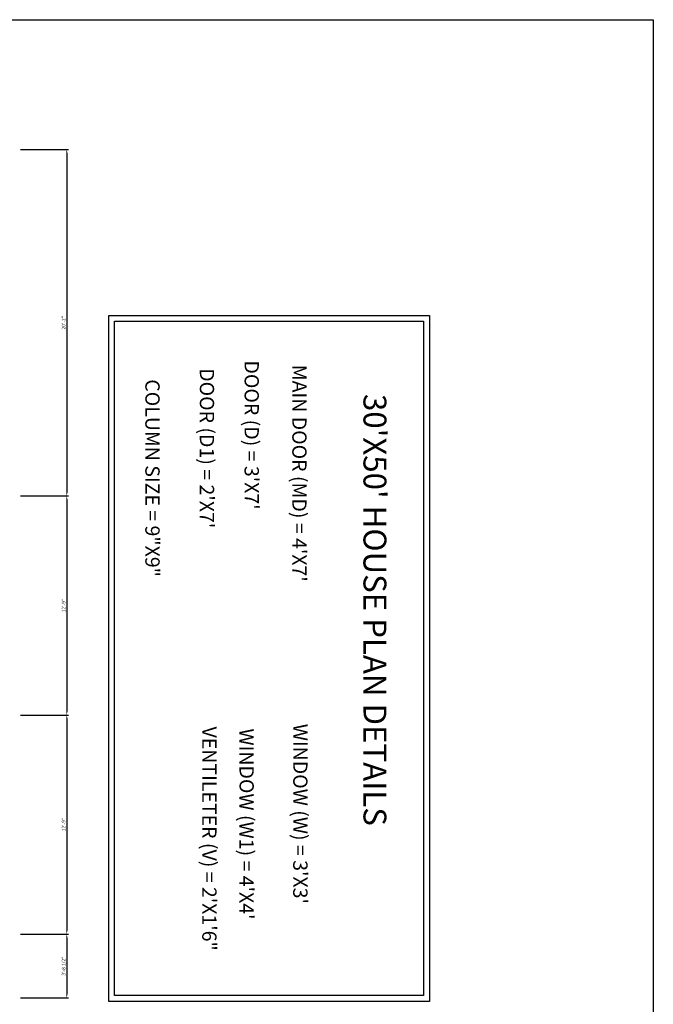
# Model space of a CAD drawing. Units: inches. Extents: x 2163 to 7246, y 928 to 2098.
# Tile 10 of 15: x 3191 to 3633, y 1411 to 2098. Entities that reach past the tile are written whole.
import ezdxf

# ---------------------------------------------------------------- set-up
doc = ezdxf.new("R2010")
doc.units = ezdxf.units.IN
for name, color, linetype, lineweight in [('A-ANNO-DIMS', 4, 'Continuous', 18), ('A-ANNO-TEXT', 7, 'Continuous', 18), ('A-ANNO-TITL', 4, 'Continuous', 30), ('A-ANNO-TTLB', 7, 'Continuous', 30)]:
    doc.layers.add(name, color=color, linetype=linetype, lineweight=lineweight)
doc.styles.get("Standard").update_dxf_attribs({"font": 'arial.ttf'})
doc.dimstyles.new('ISO-25', dxfattribs={"dimtxt": 2.5, "dimasz": 2.5, "dimexe": 1.25, "dimexo": 0.625, "dimtad": 1, "dimdec": 0, "dimlunit": 3, "dimtxsty": 'Standard', "dimcen": 2.5, "dimadec": 0, "dimazin": 0, "dimtfac": 1, "dimtdec": 0, "dimtmove": 0, "dimatfit": 3, "dimfxl": 1, "dimarcsym": 0})

# ---------------------------------------------------------------- blocks, each defined once
blk = doc.blocks.new('*D86')
at = {"layer": 'A-ANNO-DIMS', "color": 0, "lineweight": -2, "transparency": 16777216}
for p, q in [((3191.35, 2007.57), (3224.87, 2007.57)), ((3223.62, 2005.07), (3223.62, 1768.07)), ((3191.35, 1765.57), (3224.87, 1765.57))]:
    blk.add_line(p, q, dxfattribs=at)
at = {"layer": 'A-ANNO-DIMS', "color": 0, "transparency": 16777216}
for points in [[(3223.21, 2005.07), (3224.04, 2005.07), (3223.62, 2007.57)], [(3223.21, 1768.07), (3224.04, 1768.07), (3223.62, 1765.57)]]:
    blk.add_solid(points, dxfattribs=at)
at = {"layer": 'Defpoints', "color": 0, "transparency": 16777216}
for p in [(3190.72, 2007.57), (3190.72, 1765.57), (3223.62, 1765.57)]:
    blk.add_point(p, dxfattribs=at)
at = {"layer": 'A-ANNO-DIMS', "color": 0, "transparency": 16777216, "insert": (3221.72, 1886.57), "char_height": 2.5, "attachment_point": 5, "rotation": 90}
blk.add_mtext('20\'-2"', dxfattribs=at)
blk = doc.blocks.new('*D87')
at = {"layer": 'A-ANNO-DIMS', "color": 0, "lineweight": -2, "transparency": 16777216}
for p, q in [((3191.35, 1765.57), (3224.87, 1765.57)), ((3223.62, 1763.07), (3223.62, 1615.07)), ((3191.35, 1612.57), (3224.87, 1612.57))]:
    blk.add_line(p, q, dxfattribs=at)
at = {"layer": 'A-ANNO-DIMS', "color": 0, "transparency": 16777216}
for points in [[(3223.21, 1763.07), (3224.04, 1763.07), (3223.62, 1765.57)], [(3223.21, 1615.07), (3224.04, 1615.07), (3223.62, 1612.57)]]:
    blk.add_solid(points, dxfattribs=at)
at = {"layer": 'Defpoints', "color": 0, "transparency": 16777216}
for p in [(3190.72, 1765.57), (3190.72, 1612.57), (3223.62, 1612.57)]:
    blk.add_point(p, dxfattribs=at)
at = {"layer": 'A-ANNO-DIMS', "color": 0, "transparency": 16777216, "insert": (3221.72, 1689.07), "char_height": 2.5, "attachment_point": 5, "rotation": 90}
blk.add_mtext('12\'-9"', dxfattribs=at)
blk = doc.blocks.new('*D88')
at = {"layer": 'A-ANNO-DIMS', "color": 0, "lineweight": -2, "transparency": 16777216}
for p, q in [((3191.35, 1612.57), (3224.87, 1612.57)), ((3223.62, 1610.07), (3223.62, 1462.07)), ((3191.35, 1459.57), (3224.87, 1459.57))]:
    blk.add_line(p, q, dxfattribs=at)
at = {"layer": 'A-ANNO-DIMS', "color": 0, "transparency": 16777216}
for points in [[(3223.21, 1610.07), (3224.04, 1610.07), (3223.62, 1612.57)], [(3223.21, 1462.07), (3224.04, 1462.07), (3223.62, 1459.57)]]:
    blk.add_solid(points, dxfattribs=at)
at = {"layer": 'Defpoints', "color": 0, "transparency": 16777216}
for p in [(3190.72, 1612.57), (3190.72, 1459.57), (3223.62, 1459.57)]:
    blk.add_point(p, dxfattribs=at)
at = {"layer": 'A-ANNO-DIMS', "color": 0, "transparency": 16777216, "insert": (3221.72, 1536.07), "char_height": 2.5, "attachment_point": 5, "rotation": 90}
blk.add_mtext('12\'-9"', dxfattribs=at)
blk = doc.blocks.new('*D89')
at = {"layer": 'A-ANNO-DIMS', "color": 0, "lineweight": -2, "transparency": 16777216}
for p, q in [((3191.35, 1459.57), (3224.87, 1459.57)), ((3223.62, 1457.07), (3223.62, 1417.57)), ((3191.35, 1415.07), (3224.87, 1415.07))]:
    blk.add_line(p, q, dxfattribs=at)
at = {"layer": 'A-ANNO-DIMS', "color": 0, "transparency": 16777216}
for points in [[(3223.21, 1457.07), (3224.04, 1457.07), (3223.62, 1459.57)], [(3223.21, 1417.57), (3224.04, 1417.57), (3223.62, 1415.07)]]:
    blk.add_solid(points, dxfattribs=at)
at = {"layer": 'Defpoints', "color": 0, "transparency": 16777216}
for p in [(3190.72, 1459.57), (3190.72, 1415.07), (3223.62, 1415.07)]:
    blk.add_point(p, dxfattribs=at)
at = {"layer": 'A-ANNO-DIMS', "color": 0, "transparency": 16777216, "insert": (3221.71, 1437.32), "char_height": 2.5, "attachment_point": 5, "rotation": 90}
blk.add_mtext('3\'-8 1/2"', dxfattribs=at)

msp = doc.modelspace()

# ---------------------------------------------------------------- linework, layer by layer
at = {"layer": 'A-ANNO-TTLB'}
for points in [[(2162.62, 2098.21), (3633.38, 2098.21), (3633.38, 928.48), (2162.62, 928.48)], [(3476.91, 1891.61), (3476.91, 1412.65), (3252.95, 1412.65), (3252.95, 1891.61)], [(3472.91, 1887.61), (3472.91, 1416.65), (3256.95, 1416.65), (3256.95, 1887.61)]]:
    msp.add_lwpolyline(points, close=True, dxfattribs=at)

# ---------------------------------------------------------------- texts
at = {"layer": 'A-ANNO-TEXT', "char_height": 10, "attachment_point": 1, "rotation": 270}
for s, insert in [(" DOOR (D) = 3'X7'", (3357.82, 1863.28)), (" DOOR (D1) = 2'X7'", (3326.55, 1857.86)), ("MAIN DOOR (MD) = 4'X7'", (3391.15, 1857.21)), ('COLUMN SIZE = 9"X9"', (3288.5, 1847.08)), (' VENTILETER (V) = 2\'X1\'6"', (3328.24, 1607.63)), (" WINDOW (W1) = 4'X4'", (3354.28, 1606.25)), (" WINDOW (W) = 3'X3'", (3391.8, 1609.54))]:
    msp.add_mtext_dynamic_manual_height_columns(s, width=1967.0561, gutter_width=12.5, heights=[0], dxfattribs=dict(at, insert=insert))
at = {"layer": 'A-ANNO-TITL', "insert": (3446.9, 1836.82), "char_height": 16, "attachment_point": 1, "rotation": 270}
msp.add_mtext_dynamic_manual_height_columns("30'X50' HOUSE PLAN DETAILS", width=1967.0561, gutter_width=12.5, heights=[0], dxfattribs=at)

# ---------------------------------------------------------------- dimensions: what is measured, and where the dimension line sits
at = {"layer": 'A-ANNO-DIMS'}
for base, p1, p2, picture, middle in [((3223.62, 1765.57), (3190.72, 2007.57), (3190.72, 1765.57), '*D86', (3221.72, 1886.57)), ((3223.62, 1612.57), (3190.72, 1765.57), (3190.72, 1612.57), '*D87', (3221.72, 1689.07)), ((3223.62, 1459.57), (3190.72, 1612.57), (3190.72, 1459.57), '*D88', (3221.72, 1536.07)), ((3223.62, 1415.07), (3190.72, 1459.57), (3190.72, 1415.07), '*D89', (3221.71, 1437.32))]:
    dim = msp.add_linear_dim(base=base, p1=p1, p2=p2, angle=90, dimstyle='ISO-25', override={"dimdec": 1, "dimlfac": 1, "dimrnd": 0, "dimzin": 1, "dimdsep": 46, "dimlunit": 4, "dimfrac": 2}, dxfattribs=at)
    dim.commit()
    dim.dimension.update_dxf_attribs({"geometry": picture, "text_midpoint": middle})

doc.saveas('drawing.dxf')
